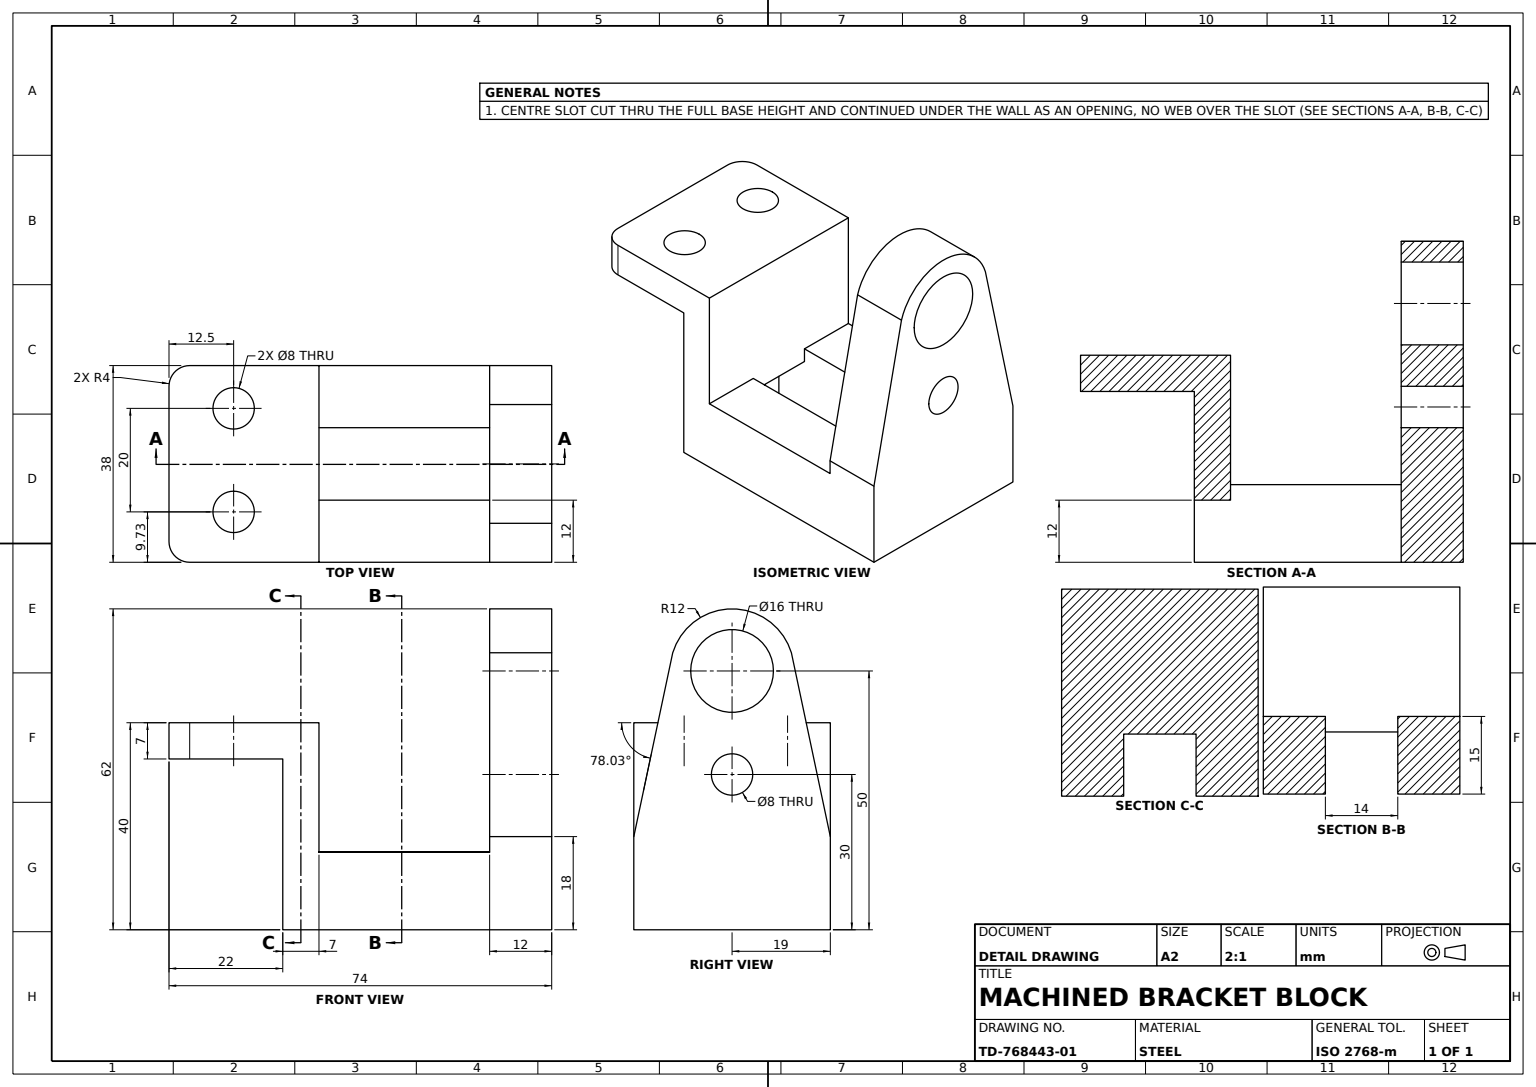
SolidWorks part; units mm, degrees
material "Plain Carbon Steel"
ref_plane "Front Plane" through (0, 0, 0) normal (0, 0, 1) x (1, 0, 0)
ref_plane "Top Plane" through (0, 0, 0) normal (0, 1, 0) x (1, 0, 0)
ref_plane "Right Plane" through (0, 0, 0) normal (1, 0, 0) x (0, 0, -1)
sketch "Base Profile Sketch" plane through (0, 0, 0) normal (0, 0, 1) x (1, 0, 0)
  line L0 (0, 0) -> (52, 0)
  line L1 (52, 0) -> (52, 18)
  line L2 (52, 18) -> (40, 18)
  line L3 (40, 18) -> (40, 8)
  line L4 (0, 0) -> (0, 18)
  line L7 (12, 8) -> (40, 8)
  line L8 (12, 8) -> (7, 8)
  line L9 (7, 8) -> (7, 18)
  line L10 (7, 18) -> (0, 18)
  dimension "D1" = 7
  dimension "D2" = 12
  dimension "D3" = 40
  dimension "D4" = 52
  dimension "D5" = 8
  dimension "D6" = 18
extrude "Base Body" add sketch "Base Profile Sketch" along normal blind 38
sketch "Upright Lug Sketch" plane through (52, 0, 0) normal (1, 0, 0) x (0, 0, -1)
  line L0 (-38, 18) -> (0, 18)
  line L1 (0, 0) -> (0, 18) construction
  line L2 (-38, 18) -> (-30.4726, 53.5185)
  line L3 (0, 18) -> (-7.5274, 53.5185)
  line L4 (-38, 18) -> (0, 18) construction
  arc A0 (-7.5274, 53.5185) -> (-30.4726, 53.5185) centre (-19, 50) ccw
  dimension "D1" = 24
  dimension "D2" = 12
  dimension "D3" = 7.5274
  dimension "D4" = 32
extrude "Upright Lug" add sketch "Upright Lug Sketch" against normal blind 12
sketch "Centre Slot Sketch" plane through (0, 0, 0) normal (-1, 0, 0) x (0, 0, 1)
  line L1 (38, 0) -> (0, 0) construction
  line L3 (26, 0) -> (26, 12)
  line L4 (26, 12) -> (12, 12)
  line L5 (12, 12) -> (12, 0)
  line L6 (0, 18) -> (0, 0) construction
  dimension "D1" = 12
  dimension "D2" = 26
  dimension "D3" = 12
extrude "Centre Slot Cut" cut sketch "Centre Slot Sketch" against normal blind 40 and the other way through all
sketch "Side Wall Sketch" plane through (0, 0, 38) normal (0, 0, 1) x (1, 0, 0)
  line L0 (0, 18) -> (0, 40)
  line L1 (7, 18) -> (7, 40)
  line L2 (7, 40) -> (0, 40)
  line L3 (0, 18) -> (7, 18)
  line L5 (0, 0) -> (52, 0) construction
  dimension "D1" = 40
extrude "Side Wall" add sketch "Side Wall Sketch" against normal blind 38
sketch "Top Flange Sketch" plane through (0, 40, 0) normal (0, 1, 0) x (1, 0, 0)
  line L0 (0, 0) -> (-18, 0)
  line L1 (0, 0) -> (0, -38)
  line L2 (-18, -38) -> (0, -38)
  line L3 (7, 0) -> (7, -38) construction
  line L4 (-22, -4) -> (-22, -34)
  arc A0 (-18, 0) -> (-22, -4) centre (-18, -4) ccw
  arc A1 (-22, -34) -> (-18, -38) centre (-18, -34) ccw
  dimension "D1" = 8
  dimension "D2" = 8
  dimension "D3" = 4
  dimension "D4" = 29
extrude "Top Flange" add sketch "Top Flange Sketch" against normal blind 7
sketch "Slot Step Pad A Sketch" plane through (0, 8, 0) normal (0, 1, 0) x (1, 0, 0)
  line L0 (7, -26) -> (40, -26)
  line L1 (40, -26) -> (40, -38)
  line L2 (40, -38) -> (7, -38)
  line L3 (7, -38) -> (7, -26)
extrude "Slot Step Pad A" add sketch "Slot Step Pad A Sketch" along normal blind 2
sketch "Slot Step Pad B Sketch" plane through (0, 8, 0) normal (0, 1, 0) x (1, 0, 0)
  line L0 (7, 0) -> (40, 0)
  line L1 (40, 0) -> (40, -12)
  line L2 (40, -12) -> (7, -12)
  line L3 (7, 0) -> (7, -38) construction
  line L4 (40, -12) -> (7, -12) construction
  line L5 (7, -12) -> (7, 0)
extrude "Slot Step Pad B" add sketch "Slot Step Pad B Sketch" along normal blind 2
sketch "Flange Holes Sketch" plane through (0, 40, 0) normal (0, 1, 0) x (1, 0, 0)
  line L1 (-22, -4) -> (-22, -34) construction
  line L2 (7, 0) -> (-18, 0) construction
  circle A0 centre (-9.5, -8.2665) radius 4
  circle A1 centre (-9.5, -28.2665) radius 4
  dimension "D1" = 8
  dimension "D2" = 8
  dimension "D6" = 8
  dimension "D3" = 20
  dimension "D4" = 12.5
  dimension "D5" = 12.5
  dimension "D7" = 8.2665
extrude "Flange Holes 2xØ8" cut sketch "Flange Holes Sketch" against normal blind 7
sketch "Lug Bore Sketch" plane through (52, 0, 0) normal (1, 0, 0) x (0, 0, -1)
  circle A0 centre (-19, 50) radius 8
  dimension "D1" = 16
  dimension "D2" = 16
extrude "Lug Bore Ø16" cut sketch "Lug Bore Sketch" against normal blind 12
sketch "Lug Hole Sketch" plane through (52, 0, 0) normal (1, 0, 0) x (0, 0, -1)
  line L0 (-19, 50) -> (-11, 50)
  circle A0 centre (-19, 30) radius 4
  circle A1 centre (-19, 50) radius 8 construction
  dimension "D1" = 8
  dimension "D3" = 8
  dimension "D2" = 20
extrude "Lug Hole Ø8" cut sketch "Lug Hole Sketch" against normal blind 12 contours A0
sketch "Slot Step Block A Sketch" plane through (0, 10, 0) normal (0, 1, 0) x (1, 0, 0)
  line L0 (7, -26) -> (40, -26)
  line L1 (40, -26) -> (40, -38)
  line L2 (40, -38) -> (7, -38)
  line L3 (7, -38) -> (7, -26)
extrude "Slot Step Block A" add sketch "Slot Step Block A Sketch" along normal blind 5
sketch "Slot Step Block B Sketch" plane through (0, 10, 0) normal (0, 1, 0) x (1, 0, 0)
  line L0 (7, 0) -> (40, 0)
  line L1 (40, 0) -> (40, -12)
  line L2 (40, -12) -> (7, -12)
  line L3 (7, -12) -> (7, 0)
extrude "Slot Step Block B" add sketch "Slot Step Block B Sketch" along normal blind 5
